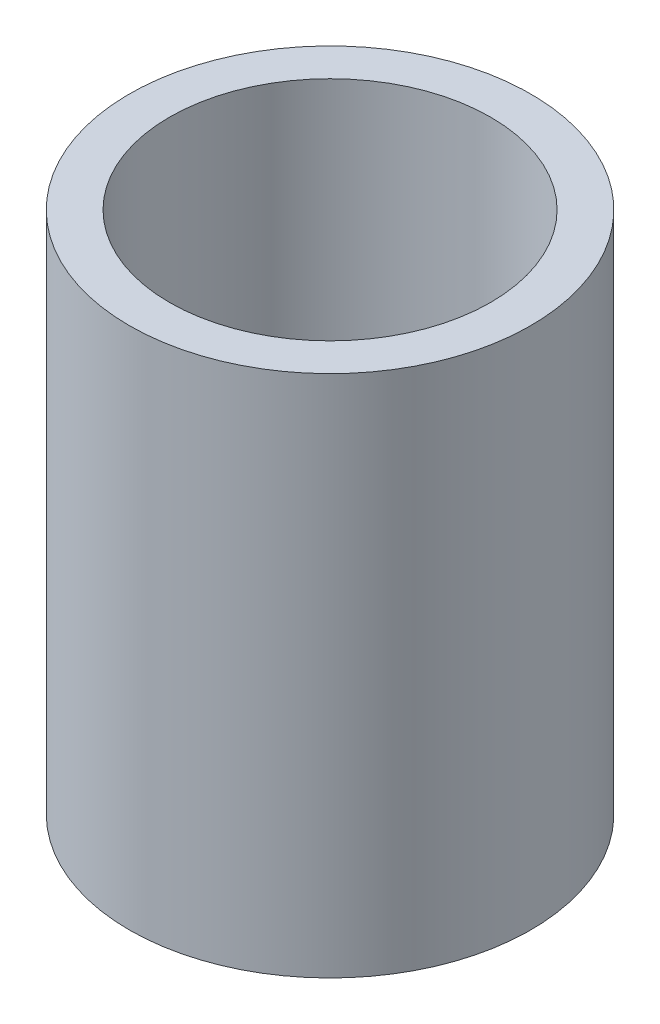
SolidWorks part; units mm, degrees
material "Plain Carbon Steel"
ref_plane "Front Plane" through (0, 0, 0) normal (0, 0, 1) x (1, 0, 0)
ref_plane "Top Plane" through (0, 0, 0) normal (0, 1, 0) x (1, 0, 0)
ref_plane "Right Plane" through (0, 0, 0) normal (1, 0, 0) x (0, 0, -1)
sketch "Tube Profile Ø125-Ø100" plane through (0, 0, 0) normal (0, 1, 0) x (1, 0, 0)
  circle A0 centre (0, 0) radius 62.5
  circle A1 centre (0, 0) radius 50
  dimension "D1" = 125
  dimension "D2" = 100
extrude "Spacer Tube L163" add sketch "Tube Profile Ø125-Ø100" along normal mid plane 163
